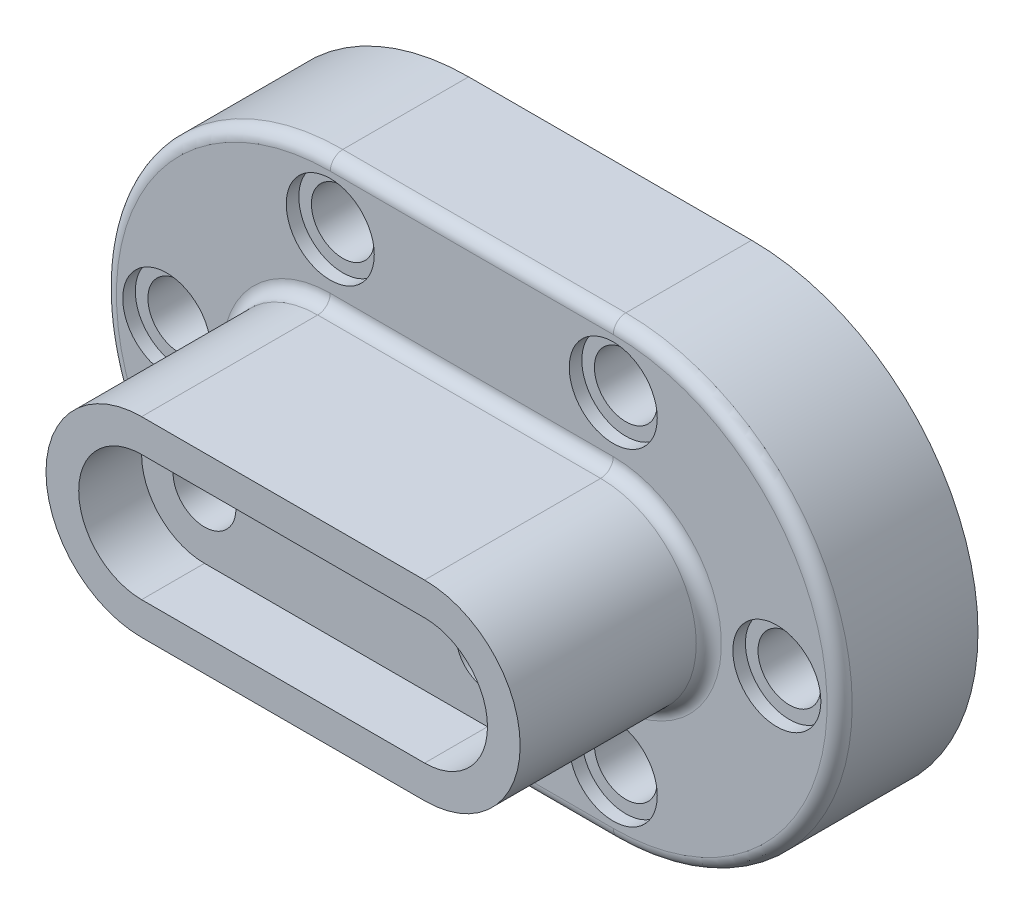
ISO-10303-21;
HEADER;
FILE_DESCRIPTION(('STEP AP214'),'2;1');
FILE_NAME('part.step','',(''),(''),'','','');
FILE_SCHEMA(('AUTOMOTIVE_DESIGN { 1 0 10303 214 1 1 1 1 }'));
ENDSEC;
DATA;
#1=APPLICATION_CONTEXT('core data for automotive mechanical design processes');
#2=APPLICATION_PROTOCOL_DEFINITION('international standard','automotive_design',2000,#1);
#3=PRODUCT_CONTEXT('',#1,'mechanical');
#4=PRODUCT('Part','Part','',(#3));
#5=PRODUCT_RELATED_PRODUCT_CATEGORY('part','',(#4));
#6=PRODUCT_DEFINITION_FORMATION('','',#4);
#7=PRODUCT_DEFINITION_CONTEXT('part definition',#1,'design');
#8=PRODUCT_DEFINITION('design','',#6,#7);
#9=PRODUCT_DEFINITION_SHAPE('','',#8);
#10=(LENGTH_UNIT() NAMED_UNIT(*) SI_UNIT(.MILLI.,.METRE.));
#11=(NAMED_UNIT(*) PLANE_ANGLE_UNIT() SI_UNIT($,.RADIAN.));
#12=(NAMED_UNIT(*) SI_UNIT($,.STERADIAN.) SOLID_ANGLE_UNIT());
#13=UNCERTAINTY_MEASURE_WITH_UNIT(LENGTH_MEASURE(1.E-05),#10,'distance_accuracy_value','');
#14=(GEOMETRIC_REPRESENTATION_CONTEXT(3) GLOBAL_UNCERTAINTY_ASSIGNED_CONTEXT((#13)) GLOBAL_UNIT_ASSIGNED_CONTEXT((#10,
#11,#12)) REPRESENTATION_CONTEXT('',''));
#15=CARTESIAN_POINT('',(0.,0.,0.));
#16=DIRECTION('',(0.,0.,1.));
#17=DIRECTION('',(1.,0.,0.));
#18=AXIS2_PLACEMENT_3D('',#15,#16,#17);
#19=CARTESIAN_POINT('',(35.508031840104,0.,0.));
#20=DIRECTION('',(0.,0.,1.));
#21=DIRECTION('',(1.,0.,0.));
#22=AXIS2_PLACEMENT_3D('',#19,#20,#21);
#23=CYLINDRICAL_SURFACE('',#22,2.5);
#24=CARTESIAN_POINT('',(35.508031840104,0.,0.));
#25=DIRECTION('',(0.,0.,1.));
#26=DIRECTION('',(1.,0.,0.));
#27=AXIS2_PLACEMENT_3D('',#24,#25,#26);
#28=CIRCLE('',#27,2.5);
#29=CARTESIAN_POINT('',(38.008031840104,0.,0.));
#30=VERTEX_POINT('',#29);
#31=EDGE_CURVE('E311',#30,#30,#28,.T.);
#32=ORIENTED_EDGE('',*,*,#31,.F.);
#33=EDGE_LOOP('',(#32));
#34=FACE_BOUND('',#33,.T.);
#35=CARTESIAN_POINT('',(35.508031840104,0.,10.));
#36=DIRECTION('',(0.,0.,1.));
#37=DIRECTION('',(1.,0.,0.));
#38=AXIS2_PLACEMENT_3D('',#35,#36,#37);
#39=CIRCLE('',#38,2.5);
#40=CARTESIAN_POINT('',(38.008031840104,0.,10.));
#41=VERTEX_POINT('',#40);
#42=EDGE_CURVE('E43',#41,#41,#39,.F.);
#43=ORIENTED_EDGE('',*,*,#42,.F.);
#44=EDGE_LOOP('',(#43));
#45=FACE_BOUND('',#44,.T.);
#46=ADVANCED_FACE('F39',(#34,#45),#23,.F.);
#47=CARTESIAN_POINT('',(-13.,0.,0.));
#48=DIRECTION('',(0.,0.,1.));
#49=DIRECTION('',(1.,0.,0.));
#50=AXIS2_PLACEMENT_3D('',#47,#48,#49);
#51=CYLINDRICAL_SURFACE('',#50,2.5);
#52=CARTESIAN_POINT('',(-13.,0.,0.));
#53=DIRECTION('',(0.,0.,1.));
#54=DIRECTION('',(1.,0.,0.));
#55=AXIS2_PLACEMENT_3D('',#52,#53,#54);
#56=CIRCLE('',#55,2.5);
#57=CARTESIAN_POINT('',(-10.5,0.,0.));
#58=VERTEX_POINT('',#57);
#59=EDGE_CURVE('E299',#58,#58,#56,.T.);
#60=ORIENTED_EDGE('',*,*,#59,.F.);
#61=EDGE_LOOP('',(#60));
#62=FACE_BOUND('',#61,.T.);
#63=CARTESIAN_POINT('',(-13.,0.,10.));
#64=DIRECTION('',(0.,0.,1.));
#65=DIRECTION('',(1.,0.,0.));
#66=AXIS2_PLACEMENT_3D('',#63,#64,#65);
#67=CIRCLE('',#66,2.5);
#68=CARTESIAN_POINT('',(-10.5,0.,10.));
#69=VERTEX_POINT('',#68);
#70=EDGE_CURVE('E304',#69,#69,#67,.F.);
#71=ORIENTED_EDGE('',*,*,#70,.F.);
#72=EDGE_LOOP('',(#71));
#73=FACE_BOUND('',#72,.T.);
#74=ADVANCED_FACE('F402',(#62,#73),#51,.F.);
#75=CARTESIAN_POINT('',(0.,13.,0.));
#76=DIRECTION('',(0.,0.,1.));
#77=DIRECTION('',(1.,0.,0.));
#78=AXIS2_PLACEMENT_3D('',#75,#76,#77);
#79=CYLINDRICAL_SURFACE('',#78,2.5);
#80=CARTESIAN_POINT('',(0.,13.,0.));
#81=DIRECTION('',(0.,0.,1.));
#82=DIRECTION('',(1.,0.,0.));
#83=AXIS2_PLACEMENT_3D('',#80,#81,#82);
#84=CIRCLE('',#83,2.5);
#85=CARTESIAN_POINT('',(2.49999999999996,13.,0.));
#86=VERTEX_POINT('',#85);
#87=EDGE_CURVE('E184',#86,#86,#84,.T.);
#88=ORIENTED_EDGE('',*,*,#87,.F.);
#89=EDGE_LOOP('',(#88));
#90=FACE_BOUND('',#89,.T.);
#91=CARTESIAN_POINT('',(0.,13.,10.));
#92=DIRECTION('',(0.,0.,1.));
#93=DIRECTION('',(1.,0.,0.));
#94=AXIS2_PLACEMENT_3D('',#91,#92,#93);
#95=CIRCLE('',#94,2.5);
#96=CARTESIAN_POINT('',(2.49999999999996,13.,10.));
#97=VERTEX_POINT('',#96);
#98=EDGE_CURVE('E248',#97,#97,#95,.F.);
#99=ORIENTED_EDGE('',*,*,#98,.F.);
#100=EDGE_LOOP('',(#99));
#101=FACE_BOUND('',#100,.T.);
#102=ADVANCED_FACE('F409',(#90,#101),#79,.F.);
#103=CARTESIAN_POINT('',(22.5,-13.,0.));
#104=DIRECTION('',(0.,0.,1.));
#105=DIRECTION('',(1.,0.,0.));
#106=AXIS2_PLACEMENT_3D('',#103,#104,#105);
#107=CYLINDRICAL_SURFACE('',#106,2.5);
#108=CARTESIAN_POINT('',(22.5,-13.,0.));
#109=DIRECTION('',(0.,0.,1.));
#110=DIRECTION('',(1.,0.,0.));
#111=AXIS2_PLACEMENT_3D('',#108,#109,#110);
#112=CIRCLE('',#111,2.5);
#113=CARTESIAN_POINT('',(25.,-13.,0.));
#114=VERTEX_POINT('',#113);
#115=EDGE_CURVE('E255',#114,#114,#112,.T.);
#116=ORIENTED_EDGE('',*,*,#115,.F.);
#117=EDGE_LOOP('',(#116));
#118=FACE_BOUND('',#117,.T.);
#119=CARTESIAN_POINT('',(22.5,-13.,10.));
#120=DIRECTION('',(0.,0.,1.));
#121=DIRECTION('',(1.,0.,0.));
#122=AXIS2_PLACEMENT_3D('',#119,#120,#121);
#123=CIRCLE('',#122,2.5);
#124=CARTESIAN_POINT('',(25.,-13.,10.));
#125=VERTEX_POINT('',#124);
#126=EDGE_CURVE('E246',#125,#125,#123,.F.);
#127=ORIENTED_EDGE('',*,*,#126,.F.);
#128=EDGE_LOOP('',(#127));
#129=FACE_BOUND('',#128,.T.);
#130=ADVANCED_FACE('F378',(#118,#129),#107,.F.);
#131=CARTESIAN_POINT('',(1.37902495690859E-13,-13.,0.));
#132=DIRECTION('',(0.,0.,1.));
#133=DIRECTION('',(1.,0.,0.));
#134=AXIS2_PLACEMENT_3D('',#131,#132,#133);
#135=CYLINDRICAL_SURFACE('',#134,2.5);
#136=CARTESIAN_POINT('',(1.37902495690859E-13,-13.,0.));
#137=DIRECTION('',(0.,0.,1.));
#138=DIRECTION('',(1.,0.,0.));
#139=AXIS2_PLACEMENT_3D('',#136,#137,#138);
#140=CIRCLE('',#139,2.5);
#141=CARTESIAN_POINT('',(2.50000000000014,-13.,0.));
#142=VERTEX_POINT('',#141);
#143=EDGE_CURVE('E366',#142,#142,#140,.T.);
#144=ORIENTED_EDGE('',*,*,#143,.F.);
#145=EDGE_LOOP('',(#144));
#146=FACE_BOUND('',#145,.T.);
#147=CARTESIAN_POINT('',(1.37902495690859E-13,-13.,10.));
#148=DIRECTION('',(0.,0.,1.));
#149=DIRECTION('',(1.,0.,0.));
#150=AXIS2_PLACEMENT_3D('',#147,#148,#149);
#151=CIRCLE('',#150,2.5);
#152=CARTESIAN_POINT('',(2.50000000000014,-13.,10.));
#153=VERTEX_POINT('',#152);
#154=EDGE_CURVE('E245',#153,#153,#151,.F.);
#155=ORIENTED_EDGE('',*,*,#154,.F.);
#156=EDGE_LOOP('',(#155));
#157=FACE_BOUND('',#156,.T.);
#158=ADVANCED_FACE('F374',(#146,#157),#135,.F.);
#159=CARTESIAN_POINT('',(22.5,13.,0.));
#160=DIRECTION('',(0.,0.,1.));
#161=DIRECTION('',(1.,0.,0.));
#162=AXIS2_PLACEMENT_3D('',#159,#160,#161);
#163=CYLINDRICAL_SURFACE('',#162,2.5);
#164=CARTESIAN_POINT('',(22.5,13.,0.));
#165=DIRECTION('',(0.,0.,1.));
#166=DIRECTION('',(1.,0.,0.));
#167=AXIS2_PLACEMENT_3D('',#164,#165,#166);
#168=CIRCLE('',#167,2.5);
#169=CARTESIAN_POINT('',(25.,13.,0.));
#170=VERTEX_POINT('',#169);
#171=EDGE_CURVE('E370',#170,#170,#168,.T.);
#172=ORIENTED_EDGE('',*,*,#171,.F.);
#173=EDGE_LOOP('',(#172));
#174=FACE_BOUND('',#173,.T.);
#175=CARTESIAN_POINT('',(22.5,13.,10.));
#176=DIRECTION('',(0.,0.,1.));
#177=DIRECTION('',(1.,0.,0.));
#178=AXIS2_PLACEMENT_3D('',#175,#176,#177);
#179=CIRCLE('',#178,2.5);
#180=CARTESIAN_POINT('',(25.,13.,10.));
#181=VERTEX_POINT('',#180);
#182=EDGE_CURVE('E237',#181,#181,#179,.F.);
#183=ORIENTED_EDGE('',*,*,#182,.F.);
#184=EDGE_LOOP('',(#183));
#185=FACE_BOUND('',#184,.T.);
#186=ADVANCED_FACE('F377',(#174,#185),#163,.F.);
#187=CARTESIAN_POINT('',(0.,0.,11.));
#188=DIRECTION('',(0.,0.,-1.));
#189=DIRECTION('',(-1.,0.,0.));
#190=AXIS2_PLACEMENT_3D('',#187,#188,#189);
#191=CYLINDRICAL_SURFACE('',#190,18.);
#192=DIRECTION('',(0.,0.,-1.));
#193=VECTOR('',#192,1.);
#194=CARTESIAN_POINT('',(0.,-18.,11.));
#195=LINE('',#194,#193);
#196=CARTESIAN_POINT('',(0.,-18.,10.));
#197=VERTEX_POINT('',#196);
#198=CARTESIAN_POINT('',(0.,-18.,0.));
#199=VERTEX_POINT('',#198);
#200=EDGE_CURVE('E236',#197,#199,#195,.T.);
#201=ORIENTED_EDGE('',*,*,#200,.F.);
#202=CARTESIAN_POINT('',(0.,0.,10.));
#203=DIRECTION('',(0.,0.,1.));
#204=DIRECTION('',(1.,0.,0.));
#205=AXIS2_PLACEMENT_3D('',#202,#203,#204);
#206=CIRCLE('',#205,18.);
#207=CARTESIAN_POINT('',(0.,18.,10.));
#208=VERTEX_POINT('',#207);
#209=EDGE_CURVE('E268',#197,#208,#206,.F.);
#210=ORIENTED_EDGE('',*,*,#209,.T.);
#211=DIRECTION('',(0.,0.,-1.));
#212=VECTOR('',#211,1.);
#213=CARTESIAN_POINT('',(0.,18.,11.));
#214=LINE('',#213,#212);
#215=CARTESIAN_POINT('',(0.,18.,0.));
#216=VERTEX_POINT('',#215);
#217=EDGE_CURVE('E229',#208,#216,#214,.T.);
#218=ORIENTED_EDGE('',*,*,#217,.T.);
#219=CARTESIAN_POINT('',(0.,0.,0.));
#220=DIRECTION('',(0.,0.,1.));
#221=DIRECTION('',(1.,0.,0.));
#222=AXIS2_PLACEMENT_3D('',#219,#220,#221);
#223=CIRCLE('',#222,18.);
#224=EDGE_CURVE('E220',#216,#199,#223,.T.);
#225=ORIENTED_EDGE('',*,*,#224,.T.);
#226=EDGE_LOOP('',(#201,#210,#218,#225));
#227=FACE_BOUND('',#226,.T.);
#228=ADVANCED_FACE('F463',(#227),#191,.T.);
#229=CARTESIAN_POINT('',(0.,-18.,11.));
#230=DIRECTION('',(0.,1.,0.));
#231=DIRECTION('',(0.,0.,1.));
#232=AXIS2_PLACEMENT_3D('',#229,#230,#231);
#233=PLANE('',#232);
#234=DIRECTION('',(0.,0.,-1.));
#235=VECTOR('',#234,1.);
#236=CARTESIAN_POINT('',(22.5,-18.,11.));
#237=LINE('',#236,#235);
#238=CARTESIAN_POINT('',(22.5,-18.,10.));
#239=VERTEX_POINT('',#238);
#240=CARTESIAN_POINT('',(22.5,-18.,0.));
#241=VERTEX_POINT('',#240);
#242=EDGE_CURVE('E234',#239,#241,#237,.T.);
#243=ORIENTED_EDGE('',*,*,#242,.F.);
#244=DIRECTION('',(1.,0.,0.));
#245=VECTOR('',#244,1.);
#246=CARTESIAN_POINT('',(0.,-18.,10.));
#247=LINE('',#246,#245);
#248=EDGE_CURVE('E48',#239,#197,#247,.F.);
#249=ORIENTED_EDGE('',*,*,#248,.T.);
#250=ORIENTED_EDGE('',*,*,#200,.T.);
#251=DIRECTION('',(1.,0.,0.));
#252=VECTOR('',#251,1.);
#253=CARTESIAN_POINT('',(0.,-18.,0.));
#254=LINE('',#253,#252);
#255=EDGE_CURVE('E222',#199,#241,#254,.T.);
#256=ORIENTED_EDGE('',*,*,#255,.T.);
#257=EDGE_LOOP('',(#243,#249,#250,#256));
#258=FACE_BOUND('',#257,.T.);
#259=ADVANCED_FACE('F512',(#258),#233,.F.);
#260=CARTESIAN_POINT('',(22.5,0.,11.));
#261=DIRECTION('',(0.,0.,-1.));
#262=DIRECTION('',(-1.,0.,0.));
#263=AXIS2_PLACEMENT_3D('',#260,#261,#262);
#264=CYLINDRICAL_SURFACE('',#263,18.);
#265=DIRECTION('',(0.,0.,-1.));
#266=VECTOR('',#265,1.);
#267=CARTESIAN_POINT('',(22.5,18.,11.));
#268=LINE('',#267,#266);
#269=CARTESIAN_POINT('',(22.5,18.,10.));
#270=VERTEX_POINT('',#269);
#271=CARTESIAN_POINT('',(22.5,18.,0.));
#272=VERTEX_POINT('',#271);
#273=EDGE_CURVE('E235',#270,#272,#268,.T.);
#274=ORIENTED_EDGE('',*,*,#273,.F.);
#275=CARTESIAN_POINT('',(22.5,0.,10.));
#276=DIRECTION('',(0.,0.,1.));
#277=DIRECTION('',(1.,0.,0.));
#278=AXIS2_PLACEMENT_3D('',#275,#276,#277);
#279=CIRCLE('',#278,18.);
#280=EDGE_CURVE('E273',#270,#239,#279,.F.);
#281=ORIENTED_EDGE('',*,*,#280,.T.);
#282=ORIENTED_EDGE('',*,*,#242,.T.);
#283=CARTESIAN_POINT('',(22.5,0.,0.));
#284=DIRECTION('',(0.,0.,1.));
#285=DIRECTION('',(1.,0.,0.));
#286=AXIS2_PLACEMENT_3D('',#283,#284,#285);
#287=CIRCLE('',#286,18.);
#288=EDGE_CURVE('E221',#241,#272,#287,.T.);
#289=ORIENTED_EDGE('',*,*,#288,.T.);
#290=EDGE_LOOP('',(#274,#281,#282,#289));
#291=FACE_BOUND('',#290,.T.);
#292=ADVANCED_FACE('F510',(#291),#264,.T.);
#293=CARTESIAN_POINT('',(0.,18.,11.));
#294=DIRECTION('',(0.,-1.,0.));
#295=DIRECTION('',(0.,0.,-1.));
#296=AXIS2_PLACEMENT_3D('',#293,#294,#295);
#297=PLANE('',#296);
#298=ORIENTED_EDGE('',*,*,#217,.F.);
#299=DIRECTION('',(-1.,0.,0.));
#300=VECTOR('',#299,1.);
#301=CARTESIAN_POINT('',(22.5,18.,10.));
#302=LINE('',#301,#300);
#303=EDGE_CURVE('E271',#208,#270,#302,.F.);
#304=ORIENTED_EDGE('',*,*,#303,.T.);
#305=ORIENTED_EDGE('',*,*,#273,.T.);
#306=DIRECTION('',(-1.,0.,0.));
#307=VECTOR('',#306,1.);
#308=CARTESIAN_POINT('',(0.,18.,0.));
#309=LINE('',#308,#307);
#310=EDGE_CURVE('E227',#272,#216,#309,.T.);
#311=ORIENTED_EDGE('',*,*,#310,.T.);
#312=EDGE_LOOP('',(#298,#304,#305,#311));
#313=FACE_BOUND('',#312,.T.);
#314=ADVANCED_FACE('F447',(#313),#297,.F.);
#315=CARTESIAN_POINT('',(0.,0.,11.));
#316=DIRECTION('',(0.,0.,1.));
#317=DIRECTION('',(1.,0.,0.));
#318=AXIS2_PLACEMENT_3D('',#315,#316,#317);
#319=PLANE('',#318);
#320=CARTESIAN_POINT('',(-13.,0.,11.));
#321=DIRECTION('',(0.,0.,1.));
#322=DIRECTION('',(1.,0.,0.));
#323=AXIS2_PLACEMENT_3D('',#320,#321,#322);
#324=CIRCLE('',#323,3.5);
#325=CARTESIAN_POINT('',(-9.5,0.,11.));
#326=VERTEX_POINT('',#325);
#327=EDGE_CURVE('E312',#326,#326,#324,.T.);
#328=ORIENTED_EDGE('',*,*,#327,.F.);
#329=EDGE_LOOP('',(#328));
#330=FACE_BOUND('',#329,.T.);
#331=CARTESIAN_POINT('',(35.508031840104,0.,11.));
#332=DIRECTION('',(0.,0.,1.));
#333=DIRECTION('',(1.,0.,0.));
#334=AXIS2_PLACEMENT_3D('',#331,#332,#333);
#335=CIRCLE('',#334,3.5);
#336=CARTESIAN_POINT('',(39.008031840104,0.,11.));
#337=VERTEX_POINT('',#336);
#338=EDGE_CURVE('E324',#337,#337,#335,.T.);
#339=ORIENTED_EDGE('',*,*,#338,.F.);
#340=EDGE_LOOP('',(#339));
#341=FACE_BOUND('',#340,.T.);
#342=DIRECTION('',(-1.,0.,0.));
#343=VECTOR('',#342,1.);
#344=CARTESIAN_POINT('',(0.,17.,11.));
#345=LINE('',#344,#343);
#346=CARTESIAN_POINT('',(22.5,17.,11.));
#347=VERTEX_POINT('',#346);
#348=CARTESIAN_POINT('',(0.,17.,11.));
#349=VERTEX_POINT('',#348);
#350=EDGE_CURVE('E262',#347,#349,#345,.T.);
#351=ORIENTED_EDGE('',*,*,#350,.T.);
#352=CARTESIAN_POINT('',(0.,0.,11.));
#353=DIRECTION('',(0.,0.,1.));
#354=DIRECTION('',(1.,0.,0.));
#355=AXIS2_PLACEMENT_3D('',#352,#353,#354);
#356=CIRCLE('',#355,17.);
#357=CARTESIAN_POINT('',(0.,-17.,11.));
#358=VERTEX_POINT('',#357);
#359=EDGE_CURVE('E270',#349,#358,#356,.T.);
#360=ORIENTED_EDGE('',*,*,#359,.T.);
#361=DIRECTION('',(1.,0.,0.));
#362=VECTOR('',#361,1.);
#363=CARTESIAN_POINT('',(22.5,-17.,11.));
#364=LINE('',#363,#362);
#365=CARTESIAN_POINT('',(22.5,-17.,11.));
#366=VERTEX_POINT('',#365);
#367=EDGE_CURVE('E264',#358,#366,#364,.T.);
#368=ORIENTED_EDGE('',*,*,#367,.T.);
#369=CARTESIAN_POINT('',(22.5,0.,11.));
#370=DIRECTION('',(0.,0.,1.));
#371=DIRECTION('',(1.,0.,0.));
#372=AXIS2_PLACEMENT_3D('',#369,#370,#371);
#373=CIRCLE('',#372,17.);
#374=EDGE_CURVE('E265',#366,#347,#373,.T.);
#375=ORIENTED_EDGE('',*,*,#374,.T.);
#376=EDGE_LOOP('',(#351,#360,#368,#375));
#377=FACE_BOUND('',#376,.T.);
#378=DIRECTION('',(1.,0.,0.));
#379=VECTOR('',#378,1.);
#380=CARTESIAN_POINT('',(0.,-8.6,11.));
#381=LINE('',#380,#379);
#382=CARTESIAN_POINT('',(22.5,-8.6,11.));
#383=VERTEX_POINT('',#382);
#384=CARTESIAN_POINT('',(0.,-8.6,11.));
#385=VERTEX_POINT('',#384);
#386=EDGE_CURVE('E238',#383,#385,#381,.F.);
#387=ORIENTED_EDGE('',*,*,#386,.T.);
#388=CARTESIAN_POINT('',(0.,0.,11.));
#389=DIRECTION('',(0.,0.,1.));
#390=DIRECTION('',(1.,0.,0.));
#391=AXIS2_PLACEMENT_3D('',#388,#389,#390);
#392=CIRCLE('',#391,8.6);
#393=CARTESIAN_POINT('',(0.,8.6,11.));
#394=VERTEX_POINT('',#393);
#395=EDGE_CURVE('E259',#385,#394,#392,.F.);
#396=ORIENTED_EDGE('',*,*,#395,.T.);
#397=DIRECTION('',(-1.,0.,0.));
#398=VECTOR('',#397,1.);
#399=CARTESIAN_POINT('',(0.,8.6,11.));
#400=LINE('',#399,#398);
#401=CARTESIAN_POINT('',(22.5,8.6,11.));
#402=VERTEX_POINT('',#401);
#403=EDGE_CURVE('E257',#394,#402,#400,.F.);
#404=ORIENTED_EDGE('',*,*,#403,.T.);
#405=CARTESIAN_POINT('',(22.5,0.,11.));
#406=DIRECTION('',(0.,0.,1.));
#407=DIRECTION('',(1.,0.,0.));
#408=AXIS2_PLACEMENT_3D('',#405,#406,#407);
#409=CIRCLE('',#408,8.6);
#410=EDGE_CURVE('E251',#402,#383,#409,.F.);
#411=ORIENTED_EDGE('',*,*,#410,.T.);
#412=EDGE_LOOP('',(#387,#396,#404,#411));
#413=FACE_BOUND('',#412,.T.);
#414=CARTESIAN_POINT('',(1.37902495690859E-13,-13.,11.));
#415=DIRECTION('',(0.,0.,1.));
#416=DIRECTION('',(1.,0.,0.));
#417=AXIS2_PLACEMENT_3D('',#414,#415,#416);
#418=CIRCLE('',#417,3.5);
#419=CARTESIAN_POINT('',(3.50000000000014,-13.,11.));
#420=VERTEX_POINT('',#419);
#421=EDGE_CURVE('E334',#420,#420,#418,.T.);
#422=ORIENTED_EDGE('',*,*,#421,.F.);
#423=EDGE_LOOP('',(#422));
#424=FACE_BOUND('',#423,.T.);
#425=CARTESIAN_POINT('',(22.5,-13.,11.));
#426=DIRECTION('',(0.,0.,1.));
#427=DIRECTION('',(1.,0.,0.));
#428=AXIS2_PLACEMENT_3D('',#425,#426,#427);
#429=CIRCLE('',#428,3.5);
#430=CARTESIAN_POINT('',(26.,-13.,11.));
#431=VERTEX_POINT('',#430);
#432=EDGE_CURVE('E355',#431,#431,#429,.T.);
#433=ORIENTED_EDGE('',*,*,#432,.F.);
#434=EDGE_LOOP('',(#433));
#435=FACE_BOUND('',#434,.T.);
#436=CARTESIAN_POINT('',(22.5,13.,11.));
#437=DIRECTION('',(0.,0.,1.));
#438=DIRECTION('',(1.,0.,0.));
#439=AXIS2_PLACEMENT_3D('',#436,#437,#438);
#440=CIRCLE('',#439,3.5);
#441=CARTESIAN_POINT('',(26.,13.,11.));
#442=VERTEX_POINT('',#441);
#443=EDGE_CURVE('E349',#442,#442,#440,.T.);
#444=ORIENTED_EDGE('',*,*,#443,.F.);
#445=EDGE_LOOP('',(#444));
#446=FACE_BOUND('',#445,.T.);
#447=CARTESIAN_POINT('',(0.,13.,11.));
#448=DIRECTION('',(0.,0.,1.));
#449=DIRECTION('',(1.,0.,0.));
#450=AXIS2_PLACEMENT_3D('',#447,#448,#449);
#451=CIRCLE('',#450,3.5);
#452=CARTESIAN_POINT('',(3.49999999999996,13.,11.));
#453=VERTEX_POINT('',#452);
#454=EDGE_CURVE('E343',#453,#453,#451,.T.);
#455=ORIENTED_EDGE('',*,*,#454,.F.);
#456=EDGE_LOOP('',(#455));
#457=FACE_BOUND('',#456,.T.);
#458=ADVANCED_FACE('F442',(#330,#341,#377,#413,#424,#435,#446,#457),#319,.T.);
#459=CARTESIAN_POINT('',(0.,0.,0.));
#460=DIRECTION('',(0.,0.,1.));
#461=DIRECTION('',(1.,0.,0.));
#462=AXIS2_PLACEMENT_3D('',#459,#460,#461);
#463=PLANE('',#462);
#464=ORIENTED_EDGE('',*,*,#59,.T.);
#465=EDGE_LOOP('',(#464));
#466=FACE_BOUND('',#465,.T.);
#467=ORIENTED_EDGE('',*,*,#31,.T.);
#468=EDGE_LOOP('',(#467));
#469=FACE_BOUND('',#468,.T.);
#470=CARTESIAN_POINT('',(0.,0.,0.));
#471=DIRECTION('',(0.,0.,1.));
#472=DIRECTION('',(1.,0.,0.));
#473=AXIS2_PLACEMENT_3D('',#470,#471,#472);
#474=CIRCLE('',#473,2.5);
#475=CARTESIAN_POINT('',(2.5,0.,0.));
#476=VERTEX_POINT('',#475);
#477=EDGE_CURVE('E327',#476,#476,#474,.T.);
#478=ORIENTED_EDGE('',*,*,#477,.T.);
#479=EDGE_LOOP('',(#478));
#480=FACE_BOUND('',#479,.T.);
#481=CARTESIAN_POINT('',(22.508031840104,0.,0.));
#482=DIRECTION('',(0.,0.,1.));
#483=DIRECTION('',(1.,0.,0.));
#484=AXIS2_PLACEMENT_3D('',#481,#482,#483);
#485=CIRCLE('',#484,2.5);
#486=CARTESIAN_POINT('',(25.008031840104,0.,0.));
#487=VERTEX_POINT('',#486);
#488=EDGE_CURVE('E340',#487,#487,#485,.T.);
#489=ORIENTED_EDGE('',*,*,#488,.T.);
#490=EDGE_LOOP('',(#489));
#491=FACE_BOUND('',#490,.T.);
#492=ORIENTED_EDGE('',*,*,#171,.T.);
#493=EDGE_LOOP('',(#492));
#494=FACE_BOUND('',#493,.T.);
#495=ORIENTED_EDGE('',*,*,#143,.T.);
#496=EDGE_LOOP('',(#495));
#497=FACE_BOUND('',#496,.T.);
#498=ORIENTED_EDGE('',*,*,#115,.T.);
#499=EDGE_LOOP('',(#498));
#500=FACE_BOUND('',#499,.T.);
#501=ORIENTED_EDGE('',*,*,#87,.T.);
#502=EDGE_LOOP('',(#501));
#503=FACE_BOUND('',#502,.T.);
#504=ORIENTED_EDGE('',*,*,#224,.F.);
#505=ORIENTED_EDGE('',*,*,#310,.F.);
#506=ORIENTED_EDGE('',*,*,#288,.F.);
#507=ORIENTED_EDGE('',*,*,#255,.F.);
#508=EDGE_LOOP('',(#504,#505,#506,#507));
#509=FACE_BOUND('',#508,.T.);
#510=ADVANCED_FACE('F375',(#466,#469,#480,#491,#494,#497,#500,#503,#509),#463,.F.);
#511=CARTESIAN_POINT('',(0.,0.,26.));
#512=DIRECTION('',(0.,0.,-1.));
#513=DIRECTION('',(-1.,0.,0.));
#514=AXIS2_PLACEMENT_3D('',#511,#512,#513);
#515=CYLINDRICAL_SURFACE('',#514,7.6);
#516=DIRECTION('',(0.,0.,-1.));
#517=VECTOR('',#516,1.);
#518=CARTESIAN_POINT('',(0.,7.6,26.));
#519=LINE('',#518,#517);
#520=CARTESIAN_POINT('',(0.,7.6,26.));
#521=VERTEX_POINT('',#520);
#522=CARTESIAN_POINT('',(0.,7.6,12.));
#523=VERTEX_POINT('',#522);
#524=EDGE_CURVE('E209',#521,#523,#519,.T.);
#525=ORIENTED_EDGE('',*,*,#524,.T.);
#526=CARTESIAN_POINT('',(0.,0.,12.));
#527=DIRECTION('',(0.,0.,1.));
#528=DIRECTION('',(1.,0.,0.));
#529=AXIS2_PLACEMENT_3D('',#526,#527,#528);
#530=CIRCLE('',#529,7.6);
#531=CARTESIAN_POINT('',(0.,-7.6,12.));
#532=VERTEX_POINT('',#531);
#533=EDGE_CURVE('E280',#523,#532,#530,.T.);
#534=ORIENTED_EDGE('',*,*,#533,.T.);
#535=DIRECTION('',(0.,0.,-1.));
#536=VECTOR('',#535,1.);
#537=CARTESIAN_POINT('',(0.,-7.6,26.));
#538=LINE('',#537,#536);
#539=CARTESIAN_POINT('',(0.,-7.6,26.));
#540=VERTEX_POINT('',#539);
#541=EDGE_CURVE('E219',#540,#532,#538,.T.);
#542=ORIENTED_EDGE('',*,*,#541,.F.);
#543=CARTESIAN_POINT('',(0.,0.,26.));
#544=DIRECTION('',(0.,0.,1.));
#545=DIRECTION('',(1.,0.,0.));
#546=AXIS2_PLACEMENT_3D('',#543,#544,#545);
#547=CIRCLE('',#546,7.6);
#548=EDGE_CURVE('E196',#521,#540,#547,.T.);
#549=ORIENTED_EDGE('',*,*,#548,.F.);
#550=EDGE_LOOP('',(#525,#534,#542,#549));
#551=FACE_BOUND('',#550,.T.);
#552=ADVANCED_FACE('F497',(#551),#515,.T.);
#553=CARTESIAN_POINT('',(0.,-7.6,26.));
#554=DIRECTION('',(0.,1.,0.));
#555=DIRECTION('',(0.,0.,1.));
#556=AXIS2_PLACEMENT_3D('',#553,#554,#555);
#557=PLANE('',#556);
#558=ORIENTED_EDGE('',*,*,#541,.T.);
#559=DIRECTION('',(1.,0.,0.));
#560=VECTOR('',#559,1.);
#561=CARTESIAN_POINT('',(0.,-7.6,12.));
#562=LINE('',#561,#560);
#563=CARTESIAN_POINT('',(22.5,-7.6,12.));
#564=VERTEX_POINT('',#563);
#565=EDGE_CURVE('E11',#532,#564,#562,.T.);
#566=ORIENTED_EDGE('',*,*,#565,.T.);
#567=DIRECTION('',(0.,0.,-1.));
#568=VECTOR('',#567,1.);
#569=CARTESIAN_POINT('',(22.5,-7.6,26.));
#570=LINE('',#569,#568);
#571=CARTESIAN_POINT('',(22.5,-7.6,26.));
#572=VERTEX_POINT('',#571);
#573=EDGE_CURVE('E211',#572,#564,#570,.T.);
#574=ORIENTED_EDGE('',*,*,#573,.F.);
#575=DIRECTION('',(1.,0.,0.));
#576=VECTOR('',#575,1.);
#577=CARTESIAN_POINT('',(0.,-7.6,26.));
#578=LINE('',#577,#576);
#579=EDGE_CURVE('E204',#540,#572,#578,.T.);
#580=ORIENTED_EDGE('',*,*,#579,.F.);
#581=EDGE_LOOP('',(#558,#566,#574,#580));
#582=FACE_BOUND('',#581,.T.);
#583=ADVANCED_FACE('F496',(#582),#557,.F.);
#584=CARTESIAN_POINT('',(22.5,0.,26.));
#585=DIRECTION('',(0.,0.,-1.));
#586=DIRECTION('',(-1.,0.,0.));
#587=AXIS2_PLACEMENT_3D('',#584,#585,#586);
#588=CYLINDRICAL_SURFACE('',#587,7.6);
#589=ORIENTED_EDGE('',*,*,#573,.T.);
#590=CARTESIAN_POINT('',(22.5,0.,12.));
#591=DIRECTION('',(0.,0.,1.));
#592=DIRECTION('',(1.,0.,0.));
#593=AXIS2_PLACEMENT_3D('',#590,#591,#592);
#594=CIRCLE('',#593,7.6);
#595=CARTESIAN_POINT('',(22.5,7.6,12.));
#596=VERTEX_POINT('',#595);
#597=EDGE_CURVE('E62',#564,#596,#594,.T.);
#598=ORIENTED_EDGE('',*,*,#597,.T.);
#599=DIRECTION('',(0.,0.,-1.));
#600=VECTOR('',#599,1.);
#601=CARTESIAN_POINT('',(22.5,7.6,26.));
#602=LINE('',#601,#600);
#603=CARTESIAN_POINT('',(22.5,7.6,26.));
#604=VERTEX_POINT('',#603);
#605=EDGE_CURVE('E215',#604,#596,#602,.T.);
#606=ORIENTED_EDGE('',*,*,#605,.F.);
#607=CARTESIAN_POINT('',(22.5,0.,26.));
#608=DIRECTION('',(0.,0.,1.));
#609=DIRECTION('',(1.,0.,0.));
#610=AXIS2_PLACEMENT_3D('',#607,#608,#609);
#611=CIRCLE('',#610,7.6);
#612=EDGE_CURVE('E203',#572,#604,#611,.T.);
#613=ORIENTED_EDGE('',*,*,#612,.F.);
#614=EDGE_LOOP('',(#589,#598,#606,#613));
#615=FACE_BOUND('',#614,.T.);
#616=ADVANCED_FACE('F495',(#615),#588,.T.);
#617=CARTESIAN_POINT('',(0.,7.6,26.));
#618=DIRECTION('',(0.,-1.,0.));
#619=DIRECTION('',(0.,0.,-1.));
#620=AXIS2_PLACEMENT_3D('',#617,#618,#619);
#621=PLANE('',#620);
#622=ORIENTED_EDGE('',*,*,#605,.T.);
#623=DIRECTION('',(-1.,0.,0.));
#624=VECTOR('',#623,1.);
#625=CARTESIAN_POINT('',(0.,7.6,12.));
#626=LINE('',#625,#624);
#627=EDGE_CURVE('E278',#596,#523,#626,.T.);
#628=ORIENTED_EDGE('',*,*,#627,.T.);
#629=ORIENTED_EDGE('',*,*,#524,.F.);
#630=DIRECTION('',(-1.,0.,0.));
#631=VECTOR('',#630,1.);
#632=CARTESIAN_POINT('',(0.,7.6,26.));
#633=LINE('',#632,#631);
#634=EDGE_CURVE('E210',#604,#521,#633,.T.);
#635=ORIENTED_EDGE('',*,*,#634,.F.);
#636=EDGE_LOOP('',(#622,#628,#629,#635));
#637=FACE_BOUND('',#636,.T.);
#638=ADVANCED_FACE('F486',(#637),#621,.F.);
#639=CARTESIAN_POINT('',(0.,0.,26.));
#640=DIRECTION('',(0.,0.,1.));
#641=DIRECTION('',(1.,0.,0.));
#642=AXIS2_PLACEMENT_3D('',#639,#640,#641);
#643=PLANE('',#642);
#644=CARTESIAN_POINT('',(0.,0.,26.));
#645=DIRECTION('',(0.,0.,1.));
#646=DIRECTION('',(1.,0.,0.));
#647=AXIS2_PLACEMENT_3D('',#644,#645,#646);
#648=CIRCLE('',#647,5.);
#649=CARTESIAN_POINT('',(0.,5.,26.));
#650=VERTEX_POINT('',#649);
#651=CARTESIAN_POINT('',(0.,-5.,26.));
#652=VERTEX_POINT('',#651);
#653=EDGE_CURVE('E162',#650,#652,#648,.T.);
#654=ORIENTED_EDGE('',*,*,#653,.F.);
#655=DIRECTION('',(-1.,0.,0.));
#656=VECTOR('',#655,1.);
#657=CARTESIAN_POINT('',(0.,5.,26.));
#658=LINE('',#657,#656);
#659=CARTESIAN_POINT('',(22.5,5.,26.));
#660=VERTEX_POINT('',#659);
#661=EDGE_CURVE('E177',#660,#650,#658,.T.);
#662=ORIENTED_EDGE('',*,*,#661,.F.);
#663=CARTESIAN_POINT('',(22.5,0.,26.));
#664=DIRECTION('',(0.,0.,1.));
#665=DIRECTION('',(1.,0.,0.));
#666=AXIS2_PLACEMENT_3D('',#663,#664,#665);
#667=CIRCLE('',#666,5.);
#668=CARTESIAN_POINT('',(22.5,-5.,26.));
#669=VERTEX_POINT('',#668);
#670=EDGE_CURVE('E185',#669,#660,#667,.T.);
#671=ORIENTED_EDGE('',*,*,#670,.F.);
#672=DIRECTION('',(1.,0.,0.));
#673=VECTOR('',#672,1.);
#674=CARTESIAN_POINT('',(0.,-5.,26.));
#675=LINE('',#674,#673);
#676=EDGE_CURVE('E192',#652,#669,#675,.T.);
#677=ORIENTED_EDGE('',*,*,#676,.F.);
#678=EDGE_LOOP('',(#654,#662,#671,#677));
#679=FACE_BOUND('',#678,.T.);
#680=ORIENTED_EDGE('',*,*,#548,.T.);
#681=ORIENTED_EDGE('',*,*,#579,.T.);
#682=ORIENTED_EDGE('',*,*,#612,.T.);
#683=ORIENTED_EDGE('',*,*,#634,.T.);
#684=EDGE_LOOP('',(#680,#681,#682,#683));
#685=FACE_BOUND('',#684,.T.);
#686=ADVANCED_FACE('F483',(#679,#685),#643,.T.);
#687=CARTESIAN_POINT('',(0.,0.,21.));
#688=DIRECTION('',(0.,0.,1.));
#689=DIRECTION('',(1.,0.,0.));
#690=AXIS2_PLACEMENT_3D('',#687,#688,#689);
#691=CYLINDRICAL_SURFACE('',#690,5.);
#692=ORIENTED_EDGE('',*,*,#653,.T.);
#693=DIRECTION('',(0.,0.,1.));
#694=VECTOR('',#693,1.);
#695=CARTESIAN_POINT('',(0.,-5.,21.));
#696=LINE('',#695,#694);
#697=CARTESIAN_POINT('',(0.,-5.,21.));
#698=VERTEX_POINT('',#697);
#699=EDGE_CURVE('E152',#698,#652,#696,.T.);
#700=ORIENTED_EDGE('',*,*,#699,.F.);
#701=CARTESIAN_POINT('',(0.,0.,21.));
#702=DIRECTION('',(0.,0.,1.));
#703=DIRECTION('',(1.,0.,0.));
#704=AXIS2_PLACEMENT_3D('',#701,#702,#703);
#705=CIRCLE('',#704,5.);
#706=CARTESIAN_POINT('',(0.,5.,21.));
#707=VERTEX_POINT('',#706);
#708=EDGE_CURVE('E156',#707,#698,#705,.T.);
#709=ORIENTED_EDGE('',*,*,#708,.F.);
#710=DIRECTION('',(0.,0.,1.));
#711=VECTOR('',#710,1.);
#712=CARTESIAN_POINT('',(0.,5.,21.));
#713=LINE('',#712,#711);
#714=EDGE_CURVE('E193',#707,#650,#713,.T.);
#715=ORIENTED_EDGE('',*,*,#714,.T.);
#716=EDGE_LOOP('',(#692,#700,#709,#715));
#717=FACE_BOUND('',#716,.T.);
#718=ADVANCED_FACE('F160',(#717),#691,.F.);
#719=CARTESIAN_POINT('',(0.,5.,21.));
#720=DIRECTION('',(0.,1.,0.));
#721=DIRECTION('',(0.,0.,1.));
#722=AXIS2_PLACEMENT_3D('',#719,#720,#721);
#723=PLANE('',#722);
#724=ORIENTED_EDGE('',*,*,#661,.T.);
#725=ORIENTED_EDGE('',*,*,#714,.F.);
#726=DIRECTION('',(-1.,0.,0.));
#727=VECTOR('',#726,1.);
#728=CARTESIAN_POINT('',(0.,5.,21.));
#729=LINE('',#728,#727);
#730=CARTESIAN_POINT('',(22.5,5.,21.));
#731=VERTEX_POINT('',#730);
#732=EDGE_CURVE('E170',#731,#707,#729,.T.);
#733=ORIENTED_EDGE('',*,*,#732,.F.);
#734=DIRECTION('',(0.,0.,1.));
#735=VECTOR('',#734,1.);
#736=CARTESIAN_POINT('',(22.5,5.,21.));
#737=LINE('',#736,#735);
#738=EDGE_CURVE('E200',#731,#660,#737,.T.);
#739=ORIENTED_EDGE('',*,*,#738,.T.);
#740=EDGE_LOOP('',(#724,#725,#733,#739));
#741=FACE_BOUND('',#740,.T.);
#742=ADVANCED_FACE('F474',(#741),#723,.F.);
#743=CARTESIAN_POINT('',(22.5,0.,21.));
#744=DIRECTION('',(0.,0.,1.));
#745=DIRECTION('',(1.,0.,0.));
#746=AXIS2_PLACEMENT_3D('',#743,#744,#745);
#747=CYLINDRICAL_SURFACE('',#746,5.);
#748=ORIENTED_EDGE('',*,*,#670,.T.);
#749=ORIENTED_EDGE('',*,*,#738,.F.);
#750=CARTESIAN_POINT('',(22.5,0.,21.));
#751=DIRECTION('',(0.,0.,1.));
#752=DIRECTION('',(1.,0.,0.));
#753=AXIS2_PLACEMENT_3D('',#750,#751,#752);
#754=CIRCLE('',#753,5.);
#755=CARTESIAN_POINT('',(22.5,-5.,21.));
#756=VERTEX_POINT('',#755);
#757=EDGE_CURVE('E174',#756,#731,#754,.T.);
#758=ORIENTED_EDGE('',*,*,#757,.F.);
#759=DIRECTION('',(0.,0.,1.));
#760=VECTOR('',#759,1.);
#761=CARTESIAN_POINT('',(22.5,-5.,21.));
#762=LINE('',#761,#760);
#763=EDGE_CURVE('E168',#756,#669,#762,.T.);
#764=ORIENTED_EDGE('',*,*,#763,.T.);
#765=EDGE_LOOP('',(#748,#749,#758,#764));
#766=FACE_BOUND('',#765,.T.);
#767=ADVANCED_FACE('F479',(#766),#747,.F.);
#768=CARTESIAN_POINT('',(0.,-5.,21.));
#769=DIRECTION('',(0.,-1.,0.));
#770=DIRECTION('',(0.,0.,-1.));
#771=AXIS2_PLACEMENT_3D('',#768,#769,#770);
#772=PLANE('',#771);
#773=ORIENTED_EDGE('',*,*,#676,.T.);
#774=ORIENTED_EDGE('',*,*,#763,.F.);
#775=DIRECTION('',(1.,0.,0.));
#776=VECTOR('',#775,1.);
#777=CARTESIAN_POINT('',(0.,-5.,21.));
#778=LINE('',#777,#776);
#779=EDGE_CURVE('E167',#698,#756,#778,.T.);
#780=ORIENTED_EDGE('',*,*,#779,.F.);
#781=ORIENTED_EDGE('',*,*,#699,.T.);
#782=EDGE_LOOP('',(#773,#774,#780,#781));
#783=FACE_BOUND('',#782,.T.);
#784=ADVANCED_FACE('F171',(#783),#772,.F.);
#785=CARTESIAN_POINT('',(0.,0.,21.));
#786=DIRECTION('',(0.,0.,1.));
#787=DIRECTION('',(1.,0.,0.));
#788=AXIS2_PLACEMENT_3D('',#785,#786,#787);
#789=PLANE('',#788);
#790=CARTESIAN_POINT('',(0.,0.,21.));
#791=DIRECTION('',(0.,0.,1.));
#792=DIRECTION('',(1.,0.,0.));
#793=AXIS2_PLACEMENT_3D('',#790,#791,#792);
#794=CIRCLE('',#793,2.5);
#795=CARTESIAN_POINT('',(2.5,0.,21.));
#796=VERTEX_POINT('',#795);
#797=EDGE_CURVE('E331',#796,#796,#794,.T.);
#798=ORIENTED_EDGE('',*,*,#797,.F.);
#799=EDGE_LOOP('',(#798));
#800=FACE_BOUND('',#799,.T.);
#801=CARTESIAN_POINT('',(22.508031840104,0.,21.));
#802=DIRECTION('',(0.,0.,1.));
#803=DIRECTION('',(1.,0.,0.));
#804=AXIS2_PLACEMENT_3D('',#801,#802,#803);
#805=CIRCLE('',#804,2.5);
#806=CARTESIAN_POINT('',(25.008031840104,0.,21.));
#807=VERTEX_POINT('',#806);
#808=EDGE_CURVE('E294',#807,#807,#805,.T.);
#809=ORIENTED_EDGE('',*,*,#808,.F.);
#810=EDGE_LOOP('',(#809));
#811=FACE_BOUND('',#810,.T.);
#812=ORIENTED_EDGE('',*,*,#708,.T.);
#813=ORIENTED_EDGE('',*,*,#779,.T.);
#814=ORIENTED_EDGE('',*,*,#757,.T.);
#815=ORIENTED_EDGE('',*,*,#732,.T.);
#816=EDGE_LOOP('',(#812,#813,#814,#815));
#817=FACE_BOUND('',#816,.T.);
#818=ADVANCED_FACE('F180',(#800,#811,#817),#789,.T.);
#819=CARTESIAN_POINT('',(22.5,13.,10.));
#820=DIRECTION('',(0.,0.,1.));
#821=DIRECTION('',(1.,0.,0.));
#822=AXIS2_PLACEMENT_3D('',#819,#820,#821);
#823=PLANE('',#822);
#824=CARTESIAN_POINT('',(22.5,13.,10.));
#825=DIRECTION('',(0.,0.,1.));
#826=DIRECTION('',(1.,0.,0.));
#827=AXIS2_PLACEMENT_3D('',#824,#825,#826);
#828=CIRCLE('',#827,3.5);
#829=CARTESIAN_POINT('',(26.,13.,10.));
#830=VERTEX_POINT('',#829);
#831=EDGE_CURVE('E345',#830,#830,#828,.T.);
#832=ORIENTED_EDGE('',*,*,#831,.T.);
#833=EDGE_LOOP('',(#832));
#834=FACE_BOUND('',#833,.T.);
#835=ORIENTED_EDGE('',*,*,#182,.T.);
#836=EDGE_LOOP('',(#835));
#837=FACE_BOUND('',#836,.T.);
#838=ADVANCED_FACE('F397',(#834,#837),#823,.T.);
#839=CARTESIAN_POINT('',(22.5,13.,10.));
#840=DIRECTION('',(0.,0.,1.));
#841=DIRECTION('',(1.,0.,0.));
#842=AXIS2_PLACEMENT_3D('',#839,#840,#841);
#843=CYLINDRICAL_SURFACE('',#842,3.5);
#844=ORIENTED_EDGE('',*,*,#831,.F.);
#845=EDGE_LOOP('',(#844));
#846=FACE_BOUND('',#845,.T.);
#847=ORIENTED_EDGE('',*,*,#443,.T.);
#848=EDGE_LOOP('',(#847));
#849=FACE_BOUND('',#848,.T.);
#850=ADVANCED_FACE('F387',(#846,#849),#843,.F.);
#851=CARTESIAN_POINT('',(1.37902495690859E-13,-13.,10.));
#852=DIRECTION('',(0.,0.,1.));
#853=DIRECTION('',(1.,0.,0.));
#854=AXIS2_PLACEMENT_3D('',#851,#852,#853);
#855=PLANE('',#854);
#856=CARTESIAN_POINT('',(1.37902495690859E-13,-13.,10.));
#857=DIRECTION('',(0.,0.,1.));
#858=DIRECTION('',(1.,0.,0.));
#859=AXIS2_PLACEMENT_3D('',#856,#857,#858);
#860=CIRCLE('',#859,3.5);
#861=CARTESIAN_POINT('',(3.50000000000014,-13.,10.));
#862=VERTEX_POINT('',#861);
#863=EDGE_CURVE('E353',#862,#862,#860,.T.);
#864=ORIENTED_EDGE('',*,*,#863,.T.);
#865=EDGE_LOOP('',(#864));
#866=FACE_BOUND('',#865,.T.);
#867=ORIENTED_EDGE('',*,*,#154,.T.);
#868=EDGE_LOOP('',(#867));
#869=FACE_BOUND('',#868,.T.);
#870=ADVANCED_FACE('F384',(#866,#869),#855,.T.);
#871=CARTESIAN_POINT('',(1.37902495690859E-13,-13.,10.));
#872=DIRECTION('',(0.,0.,1.));
#873=DIRECTION('',(1.,0.,0.));
#874=AXIS2_PLACEMENT_3D('',#871,#872,#873);
#875=CYLINDRICAL_SURFACE('',#874,3.5);
#876=ORIENTED_EDGE('',*,*,#863,.F.);
#877=EDGE_LOOP('',(#876));
#878=FACE_BOUND('',#877,.T.);
#879=ORIENTED_EDGE('',*,*,#421,.T.);
#880=EDGE_LOOP('',(#879));
#881=FACE_BOUND('',#880,.T.);
#882=ADVANCED_FACE('F383',(#878,#881),#875,.F.);
#883=CARTESIAN_POINT('',(22.5,-13.,10.));
#884=DIRECTION('',(0.,0.,1.));
#885=DIRECTION('',(1.,0.,0.));
#886=AXIS2_PLACEMENT_3D('',#883,#884,#885);
#887=PLANE('',#886);
#888=CARTESIAN_POINT('',(22.5,-13.,10.));
#889=DIRECTION('',(0.,0.,1.));
#890=DIRECTION('',(1.,0.,0.));
#891=AXIS2_PLACEMENT_3D('',#888,#889,#890);
#892=CIRCLE('',#891,3.5);
#893=CARTESIAN_POINT('',(26.,-13.,10.));
#894=VERTEX_POINT('',#893);
#895=EDGE_CURVE('E348',#894,#894,#892,.T.);
#896=ORIENTED_EDGE('',*,*,#895,.T.);
#897=EDGE_LOOP('',(#896));
#898=FACE_BOUND('',#897,.T.);
#899=ORIENTED_EDGE('',*,*,#126,.T.);
#900=EDGE_LOOP('',(#899));
#901=FACE_BOUND('',#900,.T.);
#902=ADVANCED_FACE('F395',(#898,#901),#887,.T.);
#903=CARTESIAN_POINT('',(22.5,-13.,10.));
#904=DIRECTION('',(0.,0.,1.));
#905=DIRECTION('',(1.,0.,0.));
#906=AXIS2_PLACEMENT_3D('',#903,#904,#905);
#907=CYLINDRICAL_SURFACE('',#906,3.5);
#908=ORIENTED_EDGE('',*,*,#895,.F.);
#909=EDGE_LOOP('',(#908));
#910=FACE_BOUND('',#909,.T.);
#911=ORIENTED_EDGE('',*,*,#432,.T.);
#912=EDGE_LOOP('',(#911));
#913=FACE_BOUND('',#912,.T.);
#914=ADVANCED_FACE('F429',(#910,#913),#907,.F.);
#915=CARTESIAN_POINT('',(0.,13.,10.));
#916=DIRECTION('',(0.,0.,1.));
#917=DIRECTION('',(1.,0.,0.));
#918=AXIS2_PLACEMENT_3D('',#915,#916,#917);
#919=PLANE('',#918);
#920=CARTESIAN_POINT('',(0.,13.,10.));
#921=DIRECTION('',(0.,0.,1.));
#922=DIRECTION('',(1.,0.,0.));
#923=AXIS2_PLACEMENT_3D('',#920,#921,#922);
#924=CIRCLE('',#923,3.5);
#925=CARTESIAN_POINT('',(3.49999999999996,13.,10.));
#926=VERTEX_POINT('',#925);
#927=EDGE_CURVE('E243',#926,#926,#924,.T.);
#928=ORIENTED_EDGE('',*,*,#927,.T.);
#929=EDGE_LOOP('',(#928));
#930=FACE_BOUND('',#929,.T.);
#931=ORIENTED_EDGE('',*,*,#98,.T.);
#932=EDGE_LOOP('',(#931));
#933=FACE_BOUND('',#932,.T.);
#934=ADVANCED_FACE('F435',(#930,#933),#919,.T.);
#935=CARTESIAN_POINT('',(0.,13.,10.));
#936=DIRECTION('',(0.,0.,1.));
#937=DIRECTION('',(1.,0.,0.));
#938=AXIS2_PLACEMENT_3D('',#935,#936,#937);
#939=CYLINDRICAL_SURFACE('',#938,3.5);
#940=ORIENTED_EDGE('',*,*,#927,.F.);
#941=EDGE_LOOP('',(#940));
#942=FACE_BOUND('',#941,.T.);
#943=ORIENTED_EDGE('',*,*,#454,.T.);
#944=EDGE_LOOP('',(#943));
#945=FACE_BOUND('',#944,.T.);
#946=ADVANCED_FACE('F421',(#942,#945),#939,.F.);
#947=CARTESIAN_POINT('',(22.508031840104,0.,0.));
#948=DIRECTION('',(0.,0.,1.));
#949=DIRECTION('',(1.,0.,0.));
#950=AXIS2_PLACEMENT_3D('',#947,#948,#949);
#951=CYLINDRICAL_SURFACE('',#950,2.5);
#952=ORIENTED_EDGE('',*,*,#488,.F.);
#953=EDGE_LOOP('',(#952));
#954=FACE_BOUND('',#953,.T.);
#955=ORIENTED_EDGE('',*,*,#808,.T.);
#956=EDGE_LOOP('',(#955));
#957=FACE_BOUND('',#956,.T.);
#958=ADVANCED_FACE('F416',(#954,#957),#951,.F.);
#959=CARTESIAN_POINT('',(0.,0.,0.));
#960=DIRECTION('',(0.,0.,1.));
#961=DIRECTION('',(1.,0.,0.));
#962=AXIS2_PLACEMENT_3D('',#959,#960,#961);
#963=CYLINDRICAL_SURFACE('',#962,2.5);
#964=ORIENTED_EDGE('',*,*,#477,.F.);
#965=EDGE_LOOP('',(#964));
#966=FACE_BOUND('',#965,.T.);
#967=ORIENTED_EDGE('',*,*,#797,.T.);
#968=EDGE_LOOP('',(#967));
#969=FACE_BOUND('',#968,.T.);
#970=ADVANCED_FACE('F412',(#966,#969),#963,.F.);
#971=CARTESIAN_POINT('',(22.5,0.,10.));
#972=DIRECTION('',(0.,0.,1.));
#973=DIRECTION('',(1.,0.,0.));
#974=AXIS2_PLACEMENT_3D('',#971,#972,#973);
#975=TOROIDAL_SURFACE('',#974,17.,1.);
#976=CARTESIAN_POINT('',(22.5,-17.,10.));
#977=DIRECTION('',(-1.,0.,0.));
#978=DIRECTION('',(0.,0.,1.));
#979=AXIS2_PLACEMENT_3D('',#976,#977,#978);
#980=CIRCLE('',#979,1.);
#981=EDGE_CURVE('E286',#239,#366,#980,.T.);
#982=ORIENTED_EDGE('',*,*,#981,.F.);
#983=ORIENTED_EDGE('',*,*,#280,.F.);
#984=CARTESIAN_POINT('',(22.5,17.,10.));
#985=DIRECTION('',(-1.,0.,0.));
#986=DIRECTION('',(0.,0.,1.));
#987=AXIS2_PLACEMENT_3D('',#984,#985,#986);
#988=CIRCLE('',#987,1.);
#989=EDGE_CURVE('E292',#347,#270,#988,.T.);
#990=ORIENTED_EDGE('',*,*,#989,.F.);
#991=ORIENTED_EDGE('',*,*,#374,.F.);
#992=EDGE_LOOP('',(#982,#983,#990,#991));
#993=FACE_BOUND('',#992,.T.);
#994=ADVANCED_FACE('F419',(#993),#975,.T.);
#995=CARTESIAN_POINT('',(0.,17.,10.));
#996=DIRECTION('',(1.,0.,0.));
#997=DIRECTION('',(0.,0.,-1.));
#998=AXIS2_PLACEMENT_3D('',#995,#996,#997);
#999=CYLINDRICAL_SURFACE('',#998,1.);
#1000=ORIENTED_EDGE('',*,*,#989,.T.);
#1001=ORIENTED_EDGE('',*,*,#303,.F.);
#1002=CARTESIAN_POINT('',(0.,17.,10.));
#1003=DIRECTION('',(-1.,0.,0.));
#1004=DIRECTION('',(0.,-1.,0.));
#1005=AXIS2_PLACEMENT_3D('',#1002,#1003,#1004);
#1006=CIRCLE('',#1005,1.);
#1007=EDGE_CURVE('E287',#349,#208,#1006,.T.);
#1008=ORIENTED_EDGE('',*,*,#1007,.F.);
#1009=ORIENTED_EDGE('',*,*,#350,.F.);
#1010=EDGE_LOOP('',(#1000,#1001,#1008,#1009));
#1011=FACE_BOUND('',#1010,.T.);
#1012=ADVANCED_FACE('F527',(#1011),#999,.T.);
#1013=CARTESIAN_POINT('',(0.,-17.,10.));
#1014=DIRECTION('',(-1.,0.,0.));
#1015=DIRECTION('',(0.,0.,1.));
#1016=AXIS2_PLACEMENT_3D('',#1013,#1014,#1015);
#1017=CYLINDRICAL_SURFACE('',#1016,1.);
#1018=ORIENTED_EDGE('',*,*,#981,.T.);
#1019=ORIENTED_EDGE('',*,*,#367,.F.);
#1020=CARTESIAN_POINT('',(0.,-17.,10.));
#1021=DIRECTION('',(-1.,0.,0.));
#1022=DIRECTION('',(0.,0.,1.));
#1023=AXIS2_PLACEMENT_3D('',#1020,#1021,#1022);
#1024=CIRCLE('',#1023,1.);
#1025=EDGE_CURVE('E283',#197,#358,#1024,.T.);
#1026=ORIENTED_EDGE('',*,*,#1025,.F.);
#1027=ORIENTED_EDGE('',*,*,#248,.F.);
#1028=EDGE_LOOP('',(#1018,#1019,#1026,#1027));
#1029=FACE_BOUND('',#1028,.T.);
#1030=ADVANCED_FACE('F521',(#1029),#1017,.T.);
#1031=CARTESIAN_POINT('',(0.,0.,10.));
#1032=DIRECTION('',(0.,0.,1.));
#1033=DIRECTION('',(1.,0.,0.));
#1034=AXIS2_PLACEMENT_3D('',#1031,#1032,#1033);
#1035=TOROIDAL_SURFACE('',#1034,17.,1.);
#1036=ORIENTED_EDGE('',*,*,#1007,.T.);
#1037=ORIENTED_EDGE('',*,*,#209,.F.);
#1038=ORIENTED_EDGE('',*,*,#1025,.T.);
#1039=ORIENTED_EDGE('',*,*,#359,.F.);
#1040=EDGE_LOOP('',(#1036,#1037,#1038,#1039));
#1041=FACE_BOUND('',#1040,.T.);
#1042=ADVANCED_FACE('F516',(#1041),#1035,.T.);
#1043=CARTESIAN_POINT('',(22.5,0.,12.));
#1044=DIRECTION('',(0.,0.,1.));
#1045=DIRECTION('',(1.,0.,0.));
#1046=AXIS2_PLACEMENT_3D('',#1043,#1044,#1045);
#1047=TOROIDAL_SURFACE('',#1046,8.6,1.);
#1048=CARTESIAN_POINT('',(22.5,-8.6,12.));
#1049=DIRECTION('',(1.,0.,0.));
#1050=DIRECTION('',(0.,0.,-1.));
#1051=AXIS2_PLACEMENT_3D('',#1048,#1049,#1050);
#1052=CIRCLE('',#1051,1.);
#1053=EDGE_CURVE('E301',#383,#564,#1052,.T.);
#1054=ORIENTED_EDGE('',*,*,#1053,.F.);
#1055=ORIENTED_EDGE('',*,*,#410,.F.);
#1056=CARTESIAN_POINT('',(22.5,8.6,12.));
#1057=DIRECTION('',(1.,0.,0.));
#1058=DIRECTION('',(0.,0.,-1.));
#1059=AXIS2_PLACEMENT_3D('',#1056,#1057,#1058);
#1060=CIRCLE('',#1059,1.);
#1061=EDGE_CURVE('E290',#596,#402,#1060,.T.);
#1062=ORIENTED_EDGE('',*,*,#1061,.F.);
#1063=ORIENTED_EDGE('',*,*,#597,.F.);
#1064=EDGE_LOOP('',(#1054,#1055,#1062,#1063));
#1065=FACE_BOUND('',#1064,.T.);
#1066=ADVANCED_FACE('F41',(#1065),#1047,.F.);
#1067=CARTESIAN_POINT('',(0.,8.6,12.));
#1068=DIRECTION('',(-1.,0.,0.));
#1069=DIRECTION('',(0.,0.,1.));
#1070=AXIS2_PLACEMENT_3D('',#1067,#1068,#1069);
#1071=CYLINDRICAL_SURFACE('',#1070,1.);
#1072=ORIENTED_EDGE('',*,*,#1061,.T.);
#1073=ORIENTED_EDGE('',*,*,#403,.F.);
#1074=CARTESIAN_POINT('',(0.,8.6,12.));
#1075=DIRECTION('',(1.,0.,0.));
#1076=DIRECTION('',(0.,0.,-1.));
#1077=AXIS2_PLACEMENT_3D('',#1074,#1075,#1076);
#1078=CIRCLE('',#1077,1.);
#1079=EDGE_CURVE('E296',#523,#394,#1078,.T.);
#1080=ORIENTED_EDGE('',*,*,#1079,.F.);
#1081=ORIENTED_EDGE('',*,*,#627,.F.);
#1082=EDGE_LOOP('',(#1072,#1073,#1080,#1081));
#1083=FACE_BOUND('',#1082,.T.);
#1084=ADVANCED_FACE('F544',(#1083),#1071,.F.);
#1085=CARTESIAN_POINT('',(0.,-8.6,12.));
#1086=DIRECTION('',(1.,0.,0.));
#1087=DIRECTION('',(0.,0.,-1.));
#1088=AXIS2_PLACEMENT_3D('',#1085,#1086,#1087);
#1089=CYLINDRICAL_SURFACE('',#1088,1.);
#1090=ORIENTED_EDGE('',*,*,#1053,.T.);
#1091=ORIENTED_EDGE('',*,*,#565,.F.);
#1092=CARTESIAN_POINT('',(0.,-8.6,12.));
#1093=DIRECTION('',(1.,0.,0.));
#1094=DIRECTION('',(0.,1.,0.));
#1095=AXIS2_PLACEMENT_3D('',#1092,#1093,#1094);
#1096=CIRCLE('',#1095,1.);
#1097=EDGE_CURVE('E298',#385,#532,#1096,.T.);
#1098=ORIENTED_EDGE('',*,*,#1097,.F.);
#1099=ORIENTED_EDGE('',*,*,#386,.F.);
#1100=EDGE_LOOP('',(#1090,#1091,#1098,#1099));
#1101=FACE_BOUND('',#1100,.T.);
#1102=ADVANCED_FACE('F539',(#1101),#1089,.F.);
#1103=CARTESIAN_POINT('',(0.,0.,12.));
#1104=DIRECTION('',(0.,0.,1.));
#1105=DIRECTION('',(1.,0.,0.));
#1106=AXIS2_PLACEMENT_3D('',#1103,#1104,#1105);
#1107=TOROIDAL_SURFACE('',#1106,8.6,1.);
#1108=ORIENTED_EDGE('',*,*,#1079,.T.);
#1109=ORIENTED_EDGE('',*,*,#395,.F.);
#1110=ORIENTED_EDGE('',*,*,#1097,.T.);
#1111=ORIENTED_EDGE('',*,*,#533,.F.);
#1112=EDGE_LOOP('',(#1108,#1109,#1110,#1111));
#1113=FACE_BOUND('',#1112,.T.);
#1114=ADVANCED_FACE('F534',(#1113),#1107,.F.);
#1115=CARTESIAN_POINT('',(-13.,0.,10.));
#1116=DIRECTION('',(0.,0.,1.));
#1117=DIRECTION('',(1.,0.,0.));
#1118=AXIS2_PLACEMENT_3D('',#1115,#1116,#1117);
#1119=PLANE('',#1118);
#1120=CARTESIAN_POINT('',(-13.,0.,10.));
#1121=DIRECTION('',(0.,0.,1.));
#1122=DIRECTION('',(1.,0.,0.));
#1123=AXIS2_PLACEMENT_3D('',#1120,#1121,#1122);
#1124=CIRCLE('',#1123,3.5);
#1125=CARTESIAN_POINT('',(-9.5,0.,10.));
#1126=VERTEX_POINT('',#1125);
#1127=EDGE_CURVE('E310',#1126,#1126,#1124,.T.);
#1128=ORIENTED_EDGE('',*,*,#1127,.T.);
#1129=EDGE_LOOP('',(#1128));
#1130=FACE_BOUND('',#1129,.T.);
#1131=ORIENTED_EDGE('',*,*,#70,.T.);
#1132=EDGE_LOOP('',(#1131));
#1133=FACE_BOUND('',#1132,.T.);
#1134=ADVANCED_FACE('F540',(#1130,#1133),#1119,.T.);
#1135=CARTESIAN_POINT('',(-13.,0.,10.));
#1136=DIRECTION('',(0.,0.,1.));
#1137=DIRECTION('',(1.,0.,0.));
#1138=AXIS2_PLACEMENT_3D('',#1135,#1136,#1137);
#1139=CYLINDRICAL_SURFACE('',#1138,3.5);
#1140=ORIENTED_EDGE('',*,*,#1127,.F.);
#1141=EDGE_LOOP('',(#1140));
#1142=FACE_BOUND('',#1141,.T.);
#1143=ORIENTED_EDGE('',*,*,#327,.T.);
#1144=EDGE_LOOP('',(#1143));
#1145=FACE_BOUND('',#1144,.T.);
#1146=ADVANCED_FACE('F756',(#1142,#1145),#1139,.F.);
#1147=CARTESIAN_POINT('',(35.508031840104,0.,10.));
#1148=DIRECTION('',(0.,0.,1.));
#1149=DIRECTION('',(1.,0.,0.));
#1150=AXIS2_PLACEMENT_3D('',#1147,#1148,#1149);
#1151=PLANE('',#1150);
#1152=CARTESIAN_POINT('',(35.508031840104,0.,10.));
#1153=DIRECTION('',(0.,0.,1.));
#1154=DIRECTION('',(1.,0.,0.));
#1155=AXIS2_PLACEMENT_3D('',#1152,#1153,#1154);
#1156=CIRCLE('',#1155,3.5);
#1157=CARTESIAN_POINT('',(39.008031840104,0.,10.));
#1158=VERTEX_POINT('',#1157);
#1159=EDGE_CURVE('E319',#1158,#1158,#1156,.T.);
#1160=ORIENTED_EDGE('',*,*,#1159,.T.);
#1161=EDGE_LOOP('',(#1160));
#1162=FACE_BOUND('',#1161,.T.);
#1163=ORIENTED_EDGE('',*,*,#42,.T.);
#1164=EDGE_LOOP('',(#1163));
#1165=FACE_BOUND('',#1164,.T.);
#1166=ADVANCED_FACE('F762',(#1162,#1165),#1151,.T.);
#1167=CARTESIAN_POINT('',(35.508031840104,0.,10.));
#1168=DIRECTION('',(0.,0.,1.));
#1169=DIRECTION('',(1.,0.,0.));
#1170=AXIS2_PLACEMENT_3D('',#1167,#1168,#1169);
#1171=CYLINDRICAL_SURFACE('',#1170,3.5);
#1172=ORIENTED_EDGE('',*,*,#1159,.F.);
#1173=EDGE_LOOP('',(#1172));
#1174=FACE_BOUND('',#1173,.T.);
#1175=ORIENTED_EDGE('',*,*,#338,.T.);
#1176=EDGE_LOOP('',(#1175));
#1177=FACE_BOUND('',#1176,.T.);
#1178=ADVANCED_FACE('F774',(#1174,#1177),#1171,.F.);
#1179=CLOSED_SHELL('',(#46,#74,#102,#130,#158,#186,#228,#259,#292,#314,#458,#510,#552,#583,#616,
#638,#686,#718,#742,#767,#784,#818,#838,#850,#870,#882,#902,#914,#934,#946,#958,#970,#994,#1012,
#1030,#1042,#1066,#1084,#1102,#1114,#1134,#1146,#1166,#1178));
#1180=MANIFOLD_SOLID_BREP('B2',#1179);
#1181=ADVANCED_BREP_SHAPE_REPRESENTATION('',(#18,#1180),#14);
#1182=SHAPE_DEFINITION_REPRESENTATION(#9,#1181);
ENDSEC;
END-ISO-10303-21;
